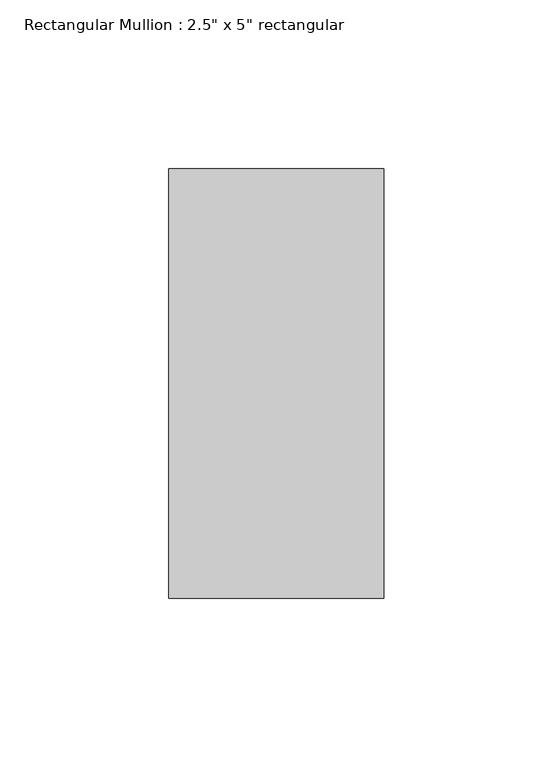
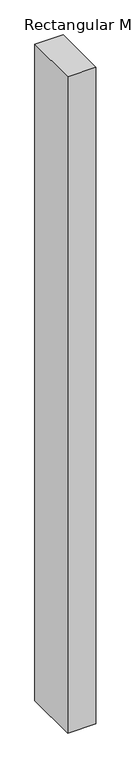
"""IFC4 building model written with IfcOpenShell, lengths in millimetres: member geometry."""

from ifc_helpers import new_model, si_unit, frame, origin, place, context, project, spatial, polyline, outline, extrude, source, transform, mapped, element, save


def member_0486e582(model_context):
    return source(origin(), model_context, "Body", "SweptSolid", [
        extrude(outline(polyline([(31.75, 63.5), (31.75, -63.5), (-31.75, -63.5), (-31.75, 63.5), (31.75, 63.5)])), frame((0.0, 0.0, -1557.3709712), z_axis=(0.0, 0.0, 1.0), x_axis=(1.0, 0.0, 0.0)), (0.0, 0.0, 1.0), 1557.3709712),
    ])


if __name__ == "__main__":
    model = new_model("IFC4")
    model_context = context("Model", 3, world=origin())
    ifc_project = project(units=[si_unit("LENGTHUNIT", "METRE", prefix="MILLI")], contexts=[model_context])
    site = spatial("IfcSite", under=ifc_project)
    building = spatial("IfcBuilding", under=site)
    placement = place(None, origin())
    member_shape = member_0486e582(model_context)
    element("IfcMember", 1, ObjectType="Rectangular Mullion : 2.5\" x 5\" rectangular", at=placement, inside=building, context=model_context, shape_type="MappedRepresentation", body=[
        mapped(member_shape, transform((0.0, 0.0, 0.0), x_axis=(1.0, 0.0, 0.0), y_axis=(0.0, 1.0, 0.0), z_axis=(0.0, 0.0, 1.0))),
    ])
    save(model, "model.ifc")

# Revit data of these elements
# Type "Rectangular Mullion : 2.5\" x 5\" rectangular"
#   built-in parameter 1007304 = 0.416667 (stored number, unit not read)
#   built-in parameter 1007301 = 0.104167 (stored number, unit not read)
#   built-in parameter 1007300 = 0.104167 (stored number, unit not read)
# Element 1 (IfcMember, "Rectangular Mullion : 2.5\" x 5\" rectangular")
#   Materials on its faces: "Aluminum"
# Materials
#   "Aluminum": class "Metal", colour RGB 247 247 247, transparency 0, Description = "Aluminum 6061", Cost = 0
